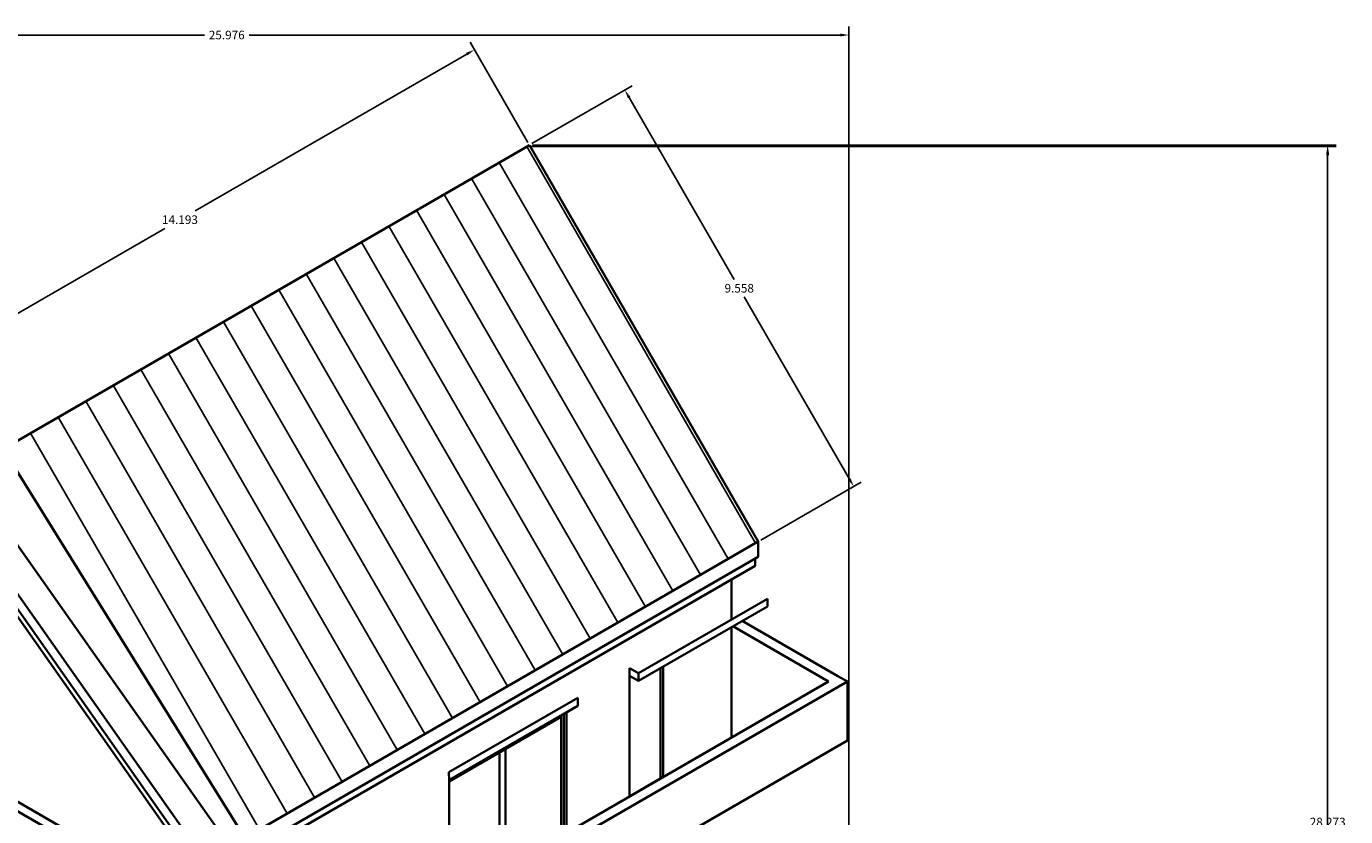
# Model space of a CAD drawing. Units: metres. Extents: x 12735 to 25554, y 20954 to 41989.
# Tile 15 of 15: x 12756 to 12784, y 20981 to 20997. Entities that reach past the tile are written whole.
import ezdxf

# ---------------------------------------------------------------- set-up
doc = ezdxf.new("R2010")
doc.units = ezdxf.units.M
doc.layers.get('Defpoints').update_dxf_attribs({"lineweight": 13})
for name, color, linetype, lineweight in [('A-ANNO-DIMS', 2, 'Continuous', 18), ('A-ELEV', 7, 'Continuous', 35), ('A-ROOF', 1, 'Continuous', 25)]:
    doc.layers.add(name, color=color, linetype=linetype, lineweight=lineweight)
doc.styles.get("Standard").update_dxf_attribs({"font": 'arial.ttf'})
doc.dimstyles.get("Standard").update_dxf_attribs({"dimtxt": 0.18, "dimasz": 0.18, "dimexe": 0.18, "dimexo": 0.0625, "dimgap": 0.09, "dimtad": 0, "dimtih": 1, "dimtoh": 1, "dimdec": 4, "dimzin": 0, "dimdsep": 46, "dimtxsty": 'Standard', "dimcen": 0.09, "dimadec": 0, "dimazin": 0, "dimtfac": 1, "dimtdec": 4, "dimtofl": 0, "dimtmove": 0, "dimatfit": 3, "dimfxl": 1, "dimtolj": 1, "dimtzin": 0, "dimarcsym": 0})

# ---------------------------------------------------------------- blocks, each defined once
blk = doc.blocks.new('*D10')
at = {"layer": 'A-ANNO-DIMS', "color": 0, "lineweight": -2, "transparency": 16777216}
for p, q in [((12766.645, 20994.825), (12783.484, 20994.825)), ((12783.304, 20994.645), (12783.304, 20975.781)), ((12783.304, 20956.553), (12783.304, 20975.417)), ((12755.849, 20956.373), (12783.484, 20956.373))]:
    blk.add_line(p, q, dxfattribs=at)
at = {"layer": 'A-ANNO-DIMS', "color": 0, "transparency": 16777216}
for points in [[(12783.274, 20994.645), (12783.334, 20994.645), (12783.304, 20994.825)], [(12783.274, 20956.553), (12783.334, 20956.553), (12783.304, 20956.373)]]:
    blk.add_solid(points, dxfattribs=at)
at = {"layer": 'Defpoints', "color": 0, "transparency": 16777216}
for p in [(12766.582, 20994.825), (12783.304, 20994.825), (12755.787, 20956.373)]:
    blk.add_point(p, dxfattribs=at)
at = {"layer": 'A-ANNO-DIMS', "color": 0, "transparency": 16777216, "insert": (12783.304, 20975.599), "char_height": 0.18, "attachment_point": 5}
blk.add_mtext('\\A1;38.45', dxfattribs=at)
blk = doc.blocks.new('*D14')
at = {"layer": 'A-ANNO-DIMS', "color": 0, "lineweight": -2, "transparency": 16777216}
for p, q in [((12766.7, 20994.856), (12783.484, 20994.856)), ((12783.304, 20994.676), (12783.304, 20980.902)), ((12783.304, 20966.764), (12783.304, 20980.538)), ((12760.589, 20966.584), (12783.484, 20966.584))]:
    blk.add_line(p, q, dxfattribs=at)
at = {"layer": 'A-ANNO-DIMS', "color": 0, "transparency": 16777216}
for points in [[(12783.274, 20994.676), (12783.334, 20994.676), (12783.304, 20994.856)], [(12783.274, 20966.764), (12783.334, 20966.764), (12783.304, 20966.584)]]:
    blk.add_solid(points, dxfattribs=at)
at = {"layer": 'Defpoints', "color": 0, "transparency": 16777216}
for p in [(12766.637, 20994.856), (12783.304, 20994.856), (12760.527, 20966.584)]:
    blk.add_point(p, dxfattribs=at)
at = {"layer": 'A-ANNO-DIMS', "color": 0, "transparency": 16777216, "insert": (12783.304, 20980.72), "char_height": 0.18, "attachment_point": 5}
blk.add_mtext('\\A1;28.273', dxfattribs=at)
blk = doc.blocks.new('*D17')
at = {"layer": 'A-ANNO-DIMS', "color": 0, "lineweight": -2, "transparency": 16777216}
for p, q in [((12766.606, 20994.911), (12765.397, 20997.004)), ((12765.331, 20996.758), (12759.656, 20993.482)), ((12753.351, 20989.842), (12759.026, 20993.118)), ((12754.314, 20987.814), (12753.105, 20989.908))]:
    blk.add_line(p, q, dxfattribs=at)
at = {"layer": 'A-ANNO-DIMS', "color": 0, "transparency": 16777216}
for points in [[(12765.316, 20996.784), (12765.346, 20996.732), (12765.487, 20996.848)], [(12753.336, 20989.868), (12753.366, 20989.816), (12753.195, 20989.752)]]:
    blk.add_solid(points, dxfattribs=at)
at = {"layer": 'Defpoints', "color": 0, "transparency": 16777216}
for p in [(12765.487, 20996.848), (12766.637, 20994.856), (12754.345, 20987.76)]:
    blk.add_point(p, dxfattribs=at)
at = {"layer": 'A-ANNO-DIMS', "color": 0, "transparency": 16777216, "insert": (12759.341, 20993.3), "char_height": 0.18, "attachment_point": 5}
blk.add_mtext('\\A1;14.193', dxfattribs=at)
blk = doc.blocks.new('*D18')
at = {"layer": 'A-ANNO-DIMS', "color": 0, "lineweight": -2, "transparency": 16777216}
for p, q in [((12766.691, 20994.888), (12768.785, 20996.096)), ((12768.719, 20995.851), (12770.913, 20992.049)), ((12773.318, 20987.884), (12771.123, 20991.686)), ((12771.47, 20986.61), (12773.564, 20987.819))]:
    blk.add_line(p, q, dxfattribs=at)
at = {"layer": 'A-ANNO-DIMS', "color": 0, "transparency": 16777216}
for points in [[(12768.745, 20995.866), (12768.693, 20995.836), (12768.629, 20996.006)], [(12773.344, 20987.899), (12773.292, 20987.869), (12773.408, 20987.729)]]:
    blk.add_solid(points, dxfattribs=at)
at = {"layer": 'Defpoints', "color": 0, "transparency": 16777216}
for p in [(12766.637, 20994.856), (12773.408, 20987.729), (12771.416, 20986.579)]:
    blk.add_point(p, dxfattribs=at)
at = {"layer": 'A-ANNO-DIMS', "color": 0, "transparency": 16777216, "insert": (12771.018, 20991.868), "char_height": 0.18, "attachment_point": 5}
blk.add_mtext('\\A1;9.558', dxfattribs=at)
blk = doc.blocks.new('*D19')
at = {"layer": 'A-ANNO-DIMS', "color": 0, "lineweight": -2, "transparency": 16777216}
for p, q in [((12747.33, 20976.079), (12747.33, 20997.336)), ((12773.306, 20974.774), (12773.306, 20997.336)), ((12747.51, 20997.156), (12759.853, 20997.156)), ((12773.126, 20997.156), (12760.783, 20997.156))]:
    blk.add_line(p, q, dxfattribs=at)
at = {"layer": 'A-ANNO-DIMS', "color": 0, "transparency": 16777216}
for points in [[(12747.51, 20997.186), (12747.51, 20997.126), (12747.33, 20997.156)], [(12773.126, 20997.186), (12773.126, 20997.126), (12773.306, 20997.156)]]:
    blk.add_solid(points, dxfattribs=at)
at = {"layer": 'Defpoints', "color": 0, "transparency": 16777216}
for p in [(12773.306, 20997.156), (12747.33, 20976.016), (12773.306, 20974.711)]:
    blk.add_point(p, dxfattribs=at)
at = {"layer": 'A-ANNO-DIMS', "color": 0, "transparency": 16777216, "insert": (12760.318, 20997.156), "char_height": 0.18, "attachment_point": 5}
blk.add_mtext('\\A1;25.976', dxfattribs=at)

msp = doc.modelspace()

# ---------------------------------------------------------------- linework, layer by layer
at = {"layer": 'A-ELEV'}
for p, q in [((12754.3454, 20987.7599), (12766.637, 20994.8564)), ((12771.4162, 20986.5786), (12766.637, 20994.8564)), ((12760.6982, 20980.3905), (12755.6472, 20988.5115)), ((12754.8551, 20988.0542), (12760.3792, 20980.2064)), ((12754.3454, 20987.7599), (12759.8695, 20979.9121)), ((12754.3454, 20987.4453), (12759.8725, 20979.5932)), ((12754.3454, 20987.2893), (12759.8695, 20979.4415)), ((12759.8695, 20979.9121), (12771.4162, 20986.5786)), ((12771.4162, 20986.5786), (12771.4162, 20986.258)), ((12759.8695, 20979.5915), (12771.4162, 20986.258)), ((12759.8695, 20979.4415), (12771.3526, 20986.0713)), ((12771.3526, 20986.0713), (12771.3526, 20986.2212)), ((12770.8601, 20984.9523), (12770.8601, 20985.7869)), ((12771.6057, 20985.3828), (12768.9125, 20983.8279)), ((12768.9125, 20983.6694), (12771.6057, 20985.2243)), ((12771.6057, 20985.3828), (12771.6057, 20985.2243)), ((12773.0797, 20983.7678), (12771.0813, 20984.9216)), ((12770.8601, 20982.4863), (12770.8601, 20984.7938)), ((12772.884, 20983.6548), (12770.8856, 20984.8086)), ((12768.9125, 20983.8279), (12768.7257, 20983.9358)), ((12768.7257, 20983.9358), (12768.7257, 20983.7772)), ((12768.9125, 20983.8279), (12768.9125, 20983.6694)), ((12769.3766, 20983.9373), (12769.3766, 20981.6298)), ((12769.4311, 20983.9688), (12769.4311, 20981.6613)), ((12765.9783, 20979.6678), (12772.884, 20983.6548)), ((12766.174, 20979.5548), (12773.2754, 20983.6548)), ((12768.7257, 20983.7772), (12768.9125, 20983.6694)), ((12768.7257, 20983.7772), (12768.7257, 20981.2541)), ((12773.2754, 20983.6548), (12773.0797, 20983.7678)), ((12773.2754, 20983.6548), (12773.2754, 20982.4199)), ((12767.6506, 20983.3141), (12764.9575, 20981.7592)), ((12767.6506, 20983.3141), (12767.6506, 20983.1492)), ((12764.963, 20981.5975), (12767.6506, 20983.1492)), ((12767.4127, 20983.0118), (12767.4127, 20980.495)), ((12764.963, 20981.566), (12767.3037, 20982.9175)), ((12767.3037, 20982.9175), (12767.3037, 20980.5579)), ((12767.3582, 20982.9804), (12767.3582, 20980.5265)), ((12766.0102, 20982.1706), (12766.0102, 20979.6853)), ((12766.1361, 20982.2434), (12766.1361, 20979.758)), ((12766.6589, 20978.5998), (12773.2754, 20982.4199)), ((12764.9575, 20981.7592), (12764.963, 20981.5975)), ((12768.7257, 20981.2541), (12769.4311, 20981.6613)), ((12755.3743, 20981.4792), (12759.8671, 20978.8853)), ((12764.963, 20981.5975), (12764.963, 20979.0807)), ((12755.3743, 20981.2792), (12759.8671, 20978.6853))]:
    msp.add_line(p, q, dxfattribs=at)
at = {"layer": 'A-ROOF'}
for p, q in [((12771.3612, 20986.5469), (12766.582, 20994.8247)), ((12770.7857, 20986.2146), (12766.0065, 20994.4924)), ((12770.2102, 20985.8823), (12765.431, 20994.1601)), ((12769.6347, 20985.55), (12764.8555, 20993.8279)), ((12769.0592, 20985.2178), (12764.28, 20993.4956)), ((12768.4836, 20984.8855), (12763.7044, 20993.1633)), ((12767.9081, 20984.5532), (12763.1289, 20992.831)), ((12767.3326, 20984.2209), (12762.5534, 20992.4988)), ((12766.7571, 20983.8887), (12761.9779, 20992.1665)), ((12766.1816, 20983.5564), (12761.4024, 20991.8342)), ((12765.6061, 20983.2241), (12760.8268, 20991.5019)), ((12765.0305, 20982.8918), (12760.2513, 20991.1697)), ((12764.455, 20982.5596), (12759.6758, 20990.8374)), ((12763.8795, 20982.2273), (12759.1003, 20990.5051)), ((12763.304, 20981.895), (12758.5248, 20990.1728)), ((12762.7285, 20981.5627), (12757.9493, 20989.8406)), ((12762.1529, 20981.2305), (12757.3737, 20989.5083)), ((12761.5774, 20980.8982), (12756.7982, 20989.176)), ((12761.0019, 20980.5659), (12756.2227, 20988.8437))]:
    msp.add_line(p, q, dxfattribs=at)

# ---------------------------------------------------------------- dimensions: what is measured, and where the dimension line sits
at = {"layer": 'A-ANNO-DIMS'}
dim = msp.add_linear_dim(base=(12773.3057, 20997.1564), p1=(12747.3297, 20976.0163), p2=(12773.3057, 20974.7113), dimstyle='Standard', override={"dimdec": 3, "dimlfac": 1, "dimrnd": 0, "dimzin": 0, "dimdsep": 46, "dimlunit": 2}, dxfattribs=at)
dim.commit()
dim.dimension.update_dxf_attribs({"geometry": '*D19', "text_midpoint": (12760.3177, 20997.1564)})
for base, p1, p2, angle, override, picture, middle in [((12765.487, 20996.8483), (12754.3454, 20987.7599), (12766.637, 20994.8564), 30, {"dimdec": 3, "dimlfac": 1, "dimrnd": 0, "dimzin": 0, "dimdsep": 46, "dimlunit": 2}, '*D17', (12759.3412, 20993.3)), ((12773.4081, 20987.7286), (12766.637, 20994.8564), (12771.4162, 20986.5786), 300, {"dimdec": 3, "dimlfac": 1, "dimrnd": 0, "dimzin": 0, "dimdsep": 46, "dimlunit": 2}, '*D18', (12771.0185, 20991.8675)), ((12783.3041, 20994.8564), (12760.5269, 20966.5835), (12766.637, 20994.8564), 90, {"dimdec": 3, "dimlfac": 1, "dimrnd": 0, "dimzin": 0, "dimdsep": 46, "dimlunit": 2}, '*D14', (12783.3041, 20980.72)), ((12783.3041, 20994.8247), (12755.7869, 20956.3734), (12766.582, 20994.8247), 90, {"dimdec": 2, "dimlfac": 1, "dimrnd": 0, "dimzin": 0, "dimdsep": 46, "dimlunit": 2}, '*D10', (12783.3041, 20975.599))]:
    dim = msp.add_linear_dim(base=base, p1=p1, p2=p2, angle=angle, dimstyle='Standard', override=override, dxfattribs=at)
    dim.commit()
    dim.dimension.update_dxf_attribs({"geometry": picture, "text_midpoint": middle})

doc.saveas('drawing.dxf')
